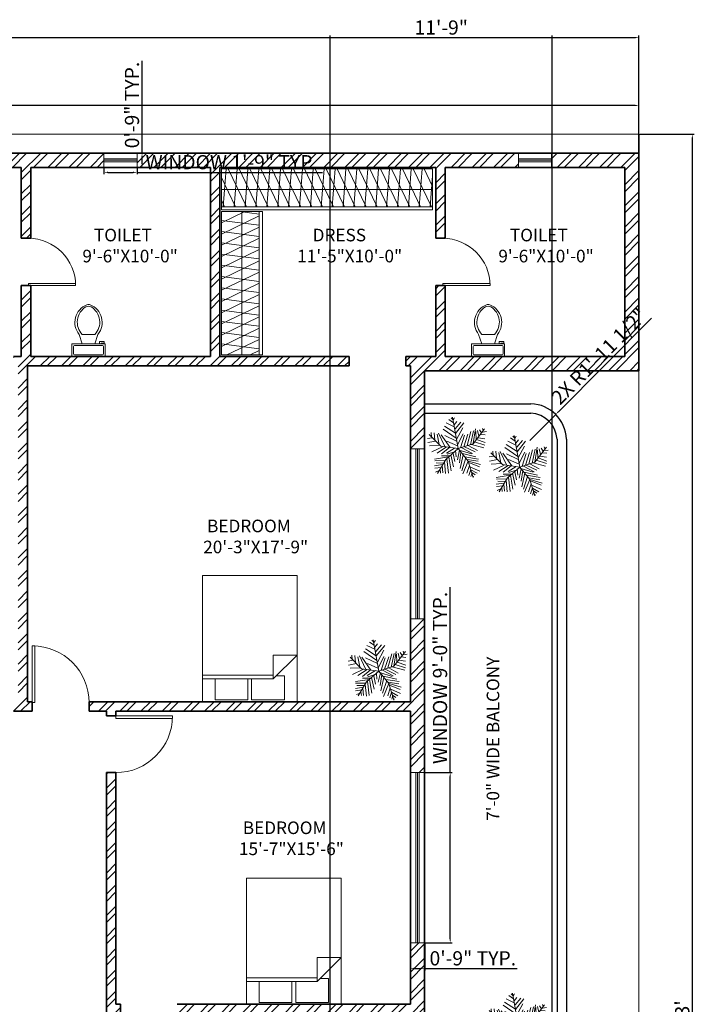
# Model space of a CAD drawing. Units: inches. Extents: x 155 to 1269, y 1260 to 2528.
# Tile 6 of 6: x 813 to 1242, y 1903 to 2528. Entities that reach past the tile are written whole.
import ezdxf

# ---------------------------------------------------------------- set-up
doc = ezdxf.new("R2010")
doc.units = ezdxf.units.IN
for name, color, linetype, lineweight in [('A-ANNO-DIMS', 2, 'Continuous', 18), ('A-AREA-IDEN', 7, 'Continuous', 18), ('A-DOOR', 3, 'Continuous', 18), ('A-FLOR-CASE', 9, 'Continuous', 18), ('A-FLOR-CASE-PATT', 252, 'Continuous', 13), ('A-FLOR-EDGE', 7, 'Continuous', 25), ('A-FLOR-FIXT', 9, 'Continuous', 18), ('A-FURN', 8, 'Continuous', 18), ('A-GLAZ', 244, 'Continuous', 18), ('A-WALL', 7, 'Continuous', 35), ('A-WALL-PATT', 252, 'Continuous', 13), ('C-PROP', 8, 'Continuous', 18), ('L-PLNT', 94, 'Continuous', 13)]:
    doc.layers.add(name, color=color, linetype=linetype, lineweight=lineweight)
doc.styles.get("Standard").update_dxf_attribs({"font": 'arial.ttf'})
doc.dimstyles.new('ISO-25', dxfattribs={"dimtxt": 9, "dimasz": 2.5, "dimexe": 1.25, "dimexo": 0.625, "dimtad": 1, "dimlunit": 3, "dimtxsty": 'Standard', "dimcen": 2.5, "dimadec": 0, "dimazin": 0, "dimtfac": 1, "dimtmove": 0, "dimatfit": 3, "dimfxl": 1, "dimarcsym": 0})

# ---------------------------------------------------------------- blocks, each defined once
blk = doc.blocks.new('*U3')
for p, q in [((0, 0), (0, -6)), ((40, 0), (40, -6))]:
    blk.add_line(p, q)
blk.add_lwpolyline([(0, 0), (0, 40), (1.75, 40), (1.75, 0)], close=True)
blk.add_arc((0, 0), 40, 0, 90)
blk = doc.blocks.new('*U4')
for p, q in [((-40, 0), (-40, 6)), ((0, 0), (0, 6))]:
    blk.add_line(p, q)
blk.add_lwpolyline([(0, 0), (0, -40), (-1.75, -40), (-1.75, 0)], close=True)
blk.add_arc((0, 0), 40, 180, 270)
blk = doc.blocks.new('*U2')
for p, q in [((0, 0), (0, -6)), ((-40, 0), (-40, -6))]:
    blk.add_line(p, q)
blk.add_lwpolyline([(0, 0), (0, 40), (-1.75, 40), (-1.75, 0)], close=True)
blk.add_arc((0, 0), 40, 90, 180)
blk = doc.blocks.new('Bed - Queen')
for p, q in [((0, -80.00003), (0, 0)), ((0, 0), (59.99999, 0)), ((59.99999, 0), (59.99999, -80.00003)), ((7.99999, -1.2), (28.79998, -1.2)), ((7.99999, -14.4), (7.99999, -1.2)), ((28.79998, -1.2), (28.79998, -14.4)), ((31.19999, -1.2), (51.99999, -1.2)), ((31.19999, -14.4), (31.19999, -1.2)), ((51.99999, -1.2), (51.99999, -16.4)), ((0, -14.4), (44.8, -14.4)), ((44.8, -16.8), (0, -16.8)), ((59.99999, -29.6), (44.8, -14.4)), ((44.8, -14.4), (44.8, -29.6)), ((51.99999, -16.4), (46.79936, -16.4)), ((44.8, -29.6), (59.99999, -29.6)), ((59.99999, -80.00003), (0, -80.00003))]:
    blk.add_line(p, q)
blk = doc.blocks.new('*U8')
for p, q in [((9.5, -6), (9.5, -2)), ((-10, -8.5), (-8, -8.5)), ((-10, -9.5), (-10, -8.5)), ((-7, -9.5), (-10, -9.5)), ((-8, -8.5), (-8, -8)), ((-7, -8), (-7, -9.5)), ((-4, -8), (-6, -14)), ((4, -8), (6, -14)), ((4, -14), (-4, -14))]:
    blk.add_line(p, q)
blk.add_lwpolyline([(10.5, -8), (10.5, 0), (-10.5, 0), (-10.5, -8)], close=True)
for points in [[(-9.5, -2), (-9.5, -6)], [(8.5, -1), (-8.5, -1)], [(-8.5, -7), (8.5, -7)]]:
    blk.add_lwpolyline(points)
for centre, radius, start, end in [((-8.62, -1.88), 0.884, 81.8699, 188.1301), ((-8.62, -6.12), 0.884, 171.8699, 278.1301), ((8.62, -1.88), 0.884, 351.8699, 98.1301), ((8.62, -6.12), 0.884, 261.8699, 8.1301), ((3.52, -21.58), 12.17, 141.46911, 247.97143), ((4.2, -21.82), 11.33, 136.36773, 238.94682), ((-3.52, -21.58), 12.17, 292.02843, 38.53071), ((-4.2, -21.82), 11.33, 301.05301, 43.63209), ((0, -27.88), 4, 245.73182, 294.26817), ((0, -29), 4, 254.86053, 285.13947)]:
    blk.add_arc(centre, radius, start, end)
blk = doc.blocks.new('*U11')
for p, q in [((-10.186, 53.64), (-13.084, 55.962)), ((0, 0), (-10.5, 57)), ((-9.099, 51.782), (-6.563, 55.962)), ((-5.114, 28.097), (-24.676, 40.636)), ((-7.288, 39.707), (-21.778, 46.673)), ((-8.737, 47.138), (-17.069, 52.711)), ((-7.65, 43.423), (-2.578, 49.46)), ((-5.839, 35.992), (4.667, 48.067)), ((-5.114, 27.632), (10.463, 46.673)), ((-2.941, 16.486), (8.652, 37.85)), ((27, 9), (48, 36)), ((27.127, 9.056), (31.112, 35.992)), ((44.153, 36.456), (45.239, 32.741)), ((-47.498, 19.737), (-55.83, 18.344)), ((-31.5, 4.5), (-52.5, 25.5)), ((-48.585, 21.131), (-49.309, 29.026)), ((-43.513, 28.561), (-42.427, 15.558)), ((-38.442, 26.239), (-34.819, 7.663)), ((-35.544, 28.097), (-24.314, 3.947)), ((-14.533, 2.09), (-30.834, 25.31)), ((-3.665, 19.273), (-27.574, 35.527)), ((-24.314, 23.917), (-2.941, 13.7)), ((-1.129, 6.734), (9.014, 26.704)), ((3.942, 1.625), (11.187, 24.381)), ((10.101, 3.483), (17.708, 26.239)), ((16.259, 5.805), (23.142, 31.348)), ((22.055, 7.198), (27.489, 32.277)), ((31.836, 30.883), (32.561, 16.486)), ((35.096, 32.741), (37.27, 22.524)), ((36.183, 19.737), (48.137, 17.88)), ((38.719, 34.134), (41.979, 28.561)), ((40.53, 25.775), (48.862, 24.846)), ((43.791, 29.954), (51.036, 30.883)), ((-40.615, 13.7), (-55.105, 10.913)), ((-33.37, 6.269), (-52.207, 5.34)), ((-28.299, 3.483), (-47.86, -5.805)), ((-21.416, 3.018), (-38.079, -8.128)), ((0, 0), (-31.5, 4.5)), ((-15.982, 2.09), (-30.11, -9.521)), ((0, 0), (-22.5, -19.5)), ((-6.563, 1.161), (-21.416, -8.128)), ((-20.691, 13.7), (-1.129, 4.876)), ((0, 0), (27, 9)), ((0, 0), (18, -22.5)), ((6.478, 1.625), (26.04, -8.592)), ((11.187, 3.483), (30.749, -5.805)), ((18.07, 5.805), (35.096, -3.483)), ((24.229, 7.663), (46.688, 1.625)), ((29.662, 12.307), (48.137, 6.269)), ((33.285, 16.486), (48.862, 10.913)), ((-17.431, -15.094), (-42.789, -18.809)), ((-15.257, -12.772), (-30.11, -12.772)), ((-6.563, -5.805), (-19.967, -9.985)), ((-17.069, -15.094), (-12.721, -40.172)), ((-13.446, -11.378), (-8.737, -32.741)), ((-9.461, -8.592), (-6.201, -23.453)), ((-4.752, -3.483), (-3.665, -14.629)), ((2.493, -3.019), (-1.491, -20.202)), ((1.769, -2.555), (24.229, -9.521)), ((5.029, -6.27), (2.131, -25.775)), ((9.014, -11.378), (3.58, -35.992)), ((14.085, -16.951), (6.478, -40.172)), ((7.565, -9.056), (32.198, -14.629)), ((12.274, -15.094), (36.907, -18.809)), ((-28.299, -29.026), (-42.789, -31.348)), ((-24.314, -21.596), (-42.427, -22.06)), ((-30.834, -34.135), (-42.427, -35.528)), ((-26.849, -26.24), (-40.253, -25.775)), ((-22.5, -19.5), (-37.5, -45)), ((-29.023, -30.884), (-27.936, -43.887)), ((-25.038, -23.918), (-22.865, -45.281)), ((-20.691, -18.345), (-17.793, -44.352)), ((18.07, -22.524), (8.289, -45.745)), ((20.244, -30.419), (15.897, -44.816)), ((16.259, -19.738), (36.183, -22.989)), ((18, -22.5), (27, -52.5)), ((18.433, -22.524), (40.53, -29.026)), ((19.157, -25.311), (38.719, -33.206)), ((21.331, -32.741), (39.081, -40.636)), ((-34.457, -39.708), (-40.978, -42.494)), ((-32.646, -36.921), (-31.921, -44.352)), ((22.78, -37.85), (19.519, -48.532)), ((22.78, -38.314), (34.372, -44.816)), ((24.591, -45.745), (23.142, -50.854)), ((24.591, -43.423), (30.749, -47.603)), ((26.764, -49.925), (28.213, -50.854))]:
    blk.add_line(p, q)
blk = doc.blocks.new('*D12')
at = {"layer": 'A-ANNO-DIMS', "color": 0, "lineweight": -2, "transparency": 16777216}
for p, q in [((227.4, 2455.81), (227.4, 2474.72)), ((1206.4, 2455.81), (1206.4, 2474.72)), ((1203.9, 2473.47), (229.9, 2473.47))]:
    blk.add_line(p, q, dxfattribs=at)
at = {"layer": 'A-ANNO-DIMS', "color": 0, "transparency": 16777216}
for points in [[(229.9, 2473.89), (229.9, 2473.06), (227.4, 2473.47)], [(1203.9, 2473.89), (1203.9, 2473.06), (1206.4, 2473.47)]]:
    blk.add_solid(points, dxfattribs=at)
at = {"layer": 'Defpoints', "color": 0, "transparency": 16777216}
for p in [(227.4, 2473.47), (227.4, 2455.18), (1206.4, 2455.18)]:
    blk.add_point(p, dxfattribs=at)
at = {"layer": 'A-ANNO-DIMS', "color": 0, "transparency": 16777216, "insert": (716.9, 2478.69), "char_height": 9, "attachment_point": 5}
blk.add_mtext('81\'-7"', dxfattribs=at)
blk = doc.blocks.new('*D13')
at = {"layer": 'A-ANNO-DIMS', "color": 0, "lineweight": -2, "transparency": 16777216}
for p, q in [((1207.02, 2455.18), (1241.52, 2455.18)), ((1240.27, 1341.68), (1240.27, 2452.68)), ((1207.02, 1339.18), (1241.52, 1339.18))]:
    blk.add_line(p, q, dxfattribs=at)
at = {"layer": 'A-ANNO-DIMS', "color": 0, "transparency": 16777216}
for points in [[(1239.85, 2452.68), (1240.68, 2452.68), (1240.27, 2455.18)], [(1239.85, 1341.68), (1240.68, 1341.68), (1240.27, 1339.18)]]:
    blk.add_solid(points, dxfattribs=at)
at = {"layer": 'Defpoints', "color": 0, "transparency": 16777216}
for p in [(1206.4, 2455.18), (1240.27, 2455.18), (1206.4, 1339.18)]:
    blk.add_point(p, dxfattribs=at)
at = {"layer": 'A-ANNO-DIMS', "color": 0, "transparency": 16777216, "insert": (1235.04, 1897.18), "char_height": 9, "attachment_point": 5, "rotation": 90}
blk.add_mtext("93'", dxfattribs=at)
blk = doc.blocks.new('WIN-21IN')
for p, q in [((21, 5.5), (0, 5.5)), ((21, 4.5), (0, 4.5)), ((21, 3.5), (0, 3.5))]:
    blk.add_line(p, q)
blk.add_lwpolyline([(0, 9), (21, 9), (21, 0), (0, 0)], close=True)
blk = doc.blocks.new('WIN-108IN')
for p, q in [((3.5, 108), (3.5, 0)), ((4.5, 108), (4.5, 0)), ((5.5, 108), (5.5, 0))]:
    blk.add_line(p, q)
blk.add_lwpolyline([(9, 108), (9, 0), (0, 0), (0, 108)], close=True)
blk = doc.blocks.new('*D24')
at = {"layer": 'A-ANNO-DIMS', "color": 0, "lineweight": -2, "transparency": 16777216}
for p, q in [((866.9, 2433.56), (866.9, 2429.78)), ((869.4, 2431.03), (885.4, 2431.03)), ((887.9, 2433.56), (887.9, 2429.78)), ((887.9, 2431.03), (1005.53, 2431.03))]:
    blk.add_line(p, q, dxfattribs=at)
at = {"layer": 'A-ANNO-DIMS', "color": 0, "transparency": 16777216}
for points in [[(869.4, 2431.45), (869.4, 2430.61), (866.9, 2431.03)], [(885.4, 2431.45), (885.4, 2430.61), (887.9, 2431.03)]]:
    blk.add_solid(points, dxfattribs=at)
at = {"layer": 'Defpoints', "color": 0, "transparency": 16777216}
for p in [(866.9, 2434.18), (887.9, 2434.18), (887.9, 2431.03)]:
    blk.add_point(p, dxfattribs=at)
at = {"layer": 'A-ANNO-DIMS', "color": 0, "transparency": 16777216, "insert": (947.97, 2436.31), "char_height": 9, "attachment_point": 5}
blk.add_mtext('WINDOW 1\'-9" TYP.', dxfattribs=at)
blk = doc.blocks.new('*D25')
at = {"layer": 'A-ANNO-DIMS', "color": 0, "lineweight": -2, "transparency": 16777216}
for p, q in [((891.05, 2443.18), (891.05, 2501.79)), ((888.52, 2443.18), (892.3, 2443.18)), ((891.05, 2436.68), (891.05, 2440.68)), ((888.52, 2434.18), (892.3, 2434.18))]:
    blk.add_line(p, q, dxfattribs=at)
at = {"layer": 'A-ANNO-DIMS', "color": 0, "transparency": 16777216}
for points in [[(890.63, 2440.68), (891.46, 2440.68), (891.05, 2443.18)], [(890.63, 2436.68), (891.46, 2436.68), (891.05, 2434.18)]]:
    blk.add_solid(points, dxfattribs=at)
at = {"layer": 'Defpoints', "color": 0, "transparency": 16777216}
for p in [(887.9, 2443.18), (891.05, 2443.18), (887.9, 2434.18)]:
    blk.add_point(p, dxfattribs=at)
at = {"layer": 'A-ANNO-DIMS', "color": 0, "transparency": 16777216, "insert": (885.83, 2473.74), "char_height": 9, "attachment_point": 5, "rotation": 90}
blk.add_mtext('0\'-9" TYP.', dxfattribs=at)
blk = doc.blocks.new('*D28')
at = {"layer": 'A-ANNO-DIMS', "color": 0, "lineweight": -2, "transparency": 16777216}
for p, q in [((1086.6, 2050.18), (1086.6, 2167.82)), ((1071.02, 2050.18), (1087.85, 2050.18)), ((1086.6, 1944.68), (1086.6, 2047.68)), ((1071.02, 1942.18), (1087.85, 1942.18))]:
    blk.add_line(p, q, dxfattribs=at)
at = {"layer": 'A-ANNO-DIMS', "color": 0, "transparency": 16777216}
for points in [[(1086.18, 2047.68), (1087.01, 2047.68), (1086.6, 2050.18)], [(1086.18, 1944.68), (1087.01, 1944.68), (1086.6, 1942.18)]]:
    blk.add_solid(points, dxfattribs=at)
at = {"layer": 'Defpoints', "color": 0, "transparency": 16777216}
for p in [(1070.4, 2050.18), (1086.6, 2050.18), (1070.4, 1942.18)]:
    blk.add_point(p, dxfattribs=at)
at = {"layer": 'A-ANNO-DIMS', "color": 0, "transparency": 16777216, "insert": (1081.32, 2110.25), "char_height": 9, "attachment_point": 5, "rotation": 90}
blk.add_mtext('WINDOW 9\'-0" TYP.', dxfattribs=at)
blk = doc.blocks.new('*D29')
at = {"layer": 'A-ANNO-DIMS', "color": 0, "lineweight": -2, "transparency": 16777216}
for p, q in [((1061.4, 1941.56), (1061.4, 1924.73)), ((1070.4, 1941.56), (1070.4, 1924.73)), ((1063.9, 1925.98), (1067.9, 1925.98)), ((1070.4, 1925.98), (1129.01, 1925.98))]:
    blk.add_line(p, q, dxfattribs=at)
at = {"layer": 'A-ANNO-DIMS', "color": 0, "transparency": 16777216}
for points in [[(1063.9, 1926.4), (1063.9, 1925.56), (1061.4, 1925.98)], [(1067.9, 1926.4), (1067.9, 1925.56), (1070.4, 1925.98)]]:
    blk.add_solid(points, dxfattribs=at)
at = {"layer": 'Defpoints', "color": 0, "transparency": 16777216}
for p in [(1061.4, 1942.18), (1070.4, 1942.18), (1070.4, 1925.98)]:
    blk.add_point(p, dxfattribs=at)
at = {"layer": 'A-ANNO-DIMS', "color": 0, "transparency": 16777216, "insert": (1100.95, 1931.2), "char_height": 9, "attachment_point": 5}
blk.add_mtext('0\'-9" TYP.', dxfattribs=at)
blk = doc.blocks.new('*D42')
at = {"layer": 'A-ANNO-DIMS', "color": 0, "lineweight": -2, "transparency": 16777216}
for p, q in [((293.4, 2443.81), (293.4, 2517.78)), ((1206.4, 2443.81), (1206.4, 2517.78)), ((295.9, 2516.53), (1203.9, 2516.53))]:
    blk.add_line(p, q, dxfattribs=at)
at = {"layer": 'A-ANNO-DIMS', "color": 0, "transparency": 16777216}
for points in [[(295.9, 2516.95), (295.9, 2516.11), (293.4, 2516.53)], [(1203.9, 2516.95), (1203.9, 2516.11), (1206.4, 2516.53)]]:
    blk.add_solid(points, dxfattribs=at)
at = {"layer": 'Defpoints', "color": 0, "transparency": 16777216}
for p in [(1206.4, 2516.53), (293.4, 2443.18), (1206.4, 2443.18)]:
    blk.add_point(p, dxfattribs=at)
at = {"layer": 'A-ANNO-DIMS', "color": 0, "transparency": 16777216, "insert": (749.9, 2521.75), "char_height": 9, "attachment_point": 5}
blk.add_mtext('76\'-1"', dxfattribs=at)
blk = doc.blocks.new('*D45')
at = {"layer": 'A-ANNO-DIMS', "color": 0, "lineweight": -2, "transparency": 16777216}
for p, q in [((1010.4, 1819.81), (1010.4, 2517.78)), ((1151.4, 1819.81), (1151.4, 2517.78)), ((1012.9, 2516.53), (1148.9, 2516.53))]:
    blk.add_line(p, q, dxfattribs=at)
at = {"layer": 'A-ANNO-DIMS', "color": 0, "transparency": 16777216}
for points in [[(1012.9, 2516.95), (1012.9, 2516.11), (1010.4, 2516.53)], [(1148.9, 2516.95), (1148.9, 2516.11), (1151.4, 2516.53)]]:
    blk.add_solid(points, dxfattribs=at)
at = {"layer": 'Defpoints', "color": 0, "transparency": 16777216}
for p in [(1151.4, 2516.53), (1010.4, 1819.18), (1151.4, 1819.18)]:
    blk.add_point(p, dxfattribs=at)
at = {"layer": 'A-ANNO-DIMS', "color": 0, "transparency": 16777216, "insert": (1080.9, 2521.75), "char_height": 9, "attachment_point": 5}
blk.add_mtext('11\'-9"', dxfattribs=at)
blk = doc.blocks.new('*D49')
at = {"layer": 'A-ANNO-DIMS', "color": 0, "lineweight": -2, "transparency": 16777216}
for p, q in [((1214.34, 2338.57), (1155.3, 2279.18)), ((1137.09, 2260.87), (1153.54, 2277.41))]:
    blk.add_line(p, q, dxfattribs=at)
at = {"layer": 'A-ANNO-DIMS', "color": 0, "transparency": 16777216}
blk.add_solid([(1155, 2279.48), (1155.6, 2278.89), (1153.54, 2277.41)], dxfattribs=at)
at = {"layer": 'Defpoints', "color": 0, "transparency": 16777216}
for p in [(1153.54, 2277.41), (1137.09, 2260.87)]:
    blk.add_point(p, dxfattribs=at)
at = {"layer": 'A-ANNO-DIMS', "color": 0, "transparency": 16777216, "insert": (1181.96, 2313.49), "char_height": 9, "attachment_point": 5, "rotation": 45.16583}
blk.add_mtext('2X R1\'-11 1/2"', dxfattribs=at)

msp = doc.modelspace()

# ---------------------------------------------------------------- hatches: boundary and pattern name
at = {"layer": 'A-FLOR-CASE-PATT'}
h = msp.add_hatch(dxfattribs=at)
h.set_pattern_fill('ANSI31', color=256, scale=1.9617, angle=70.6537, style=0)
h.paths.add_polyline_path([(941.397, 2409.181), (1075.397, 2409.181), (1075.397, 2433.181), (941.397, 2433.181)])
h = msp.add_hatch(dxfattribs=at)
h.set_pattern_fill('ANSI31', color=256, scale=2.16999, angle=40.6661, style=0)
h.paths.add_polyline_path([(941.397, 2409.181), (1075.397, 2409.181), (1075.397, 2433.181), (941.397, 2433.181)])
h = msp.add_hatch(dxfattribs=at)
h.set_pattern_fill('ANSI31', color=256, scale=2.02178, angle=-19.2697, style=0)
h.paths.add_polyline_path([(941.397, 2315.181), (965.397, 2315.181), (965.397, 2406.181), (941.397, 2406.181)])
h = msp.add_hatch(dxfattribs=at)
h.set_pattern_fill('ANSI31', color=256, scale=2.225716, angle=127.6207, style=0)
h.paths.add_polyline_path([(941.397, 2315.181), (965.397, 2315.181), (965.397, 2406.181), (941.397, 2406.181)])
at = {"layer": 'A-WALL-PATT'}
h = msp.add_hatch(dxfattribs=at)
h.set_pattern_fill('ANSI32', color=256)
h.paths.add_polyline_path([(614.897, 1534.181), (593.397, 1534.181), (593.397, 1555.181), (589.397, 1555.181), (589.397, 1534.181), (517.397, 1534.181), (517.397, 1555.181), (511.397, 1555.181), (511.397, 1495.181), (488.631, 1495.181), (488.631, 1486.181), (517.397, 1486.181), (517.397, 1525.181), (614.897, 1525.181)])
h.paths.add_polyline_path([(440.631, 1495.181), (344.954, 1495.181), (344.954, 1486.181), (440.631, 1486.181)])
h.paths.add_polyline_path([(323.954, 1495.181), (302.397, 1495.181), (302.397, 1625.863), (332.397, 1625.863), (332.397, 1631.863), (302.397, 1631.863), (302.397, 1634.984), (293.397, 1634.984), (293.397, 1486.181), (323.954, 1486.181)])
h.paths.add_polyline_path([(302.397, 1753.181), (386.397, 1753.181), (386.397, 1726.181), (392.397, 1726.181), (392.397, 1753.181), (511.397, 1753.181), (511.397, 1693.181), (392.397, 1693.181), (392.397, 1696.181), (386.397, 1696.181), (386.397, 1693.181), (368.397, 1693.181), (368.397, 1687.181), (511.397, 1687.181), (511.397, 1663.181), (517.397, 1663.181), (517.397, 1891.181), (539.397, 1891.181), (539.397, 1897.181), (517.397, 1897.181), (517.397, 2050.181), (511.397, 2050.181), (511.397, 1903.181), (374.397, 1903.181), (374.397, 1897.181), (410.397, 1897.181), (410.397, 1843.181), (416.397, 1843.181), (416.397, 1897.181), (511.397, 1897.181), (511.397, 1759.181), (416.397, 1759.181), (416.397, 1813.181), (410.397, 1813.181), (410.397, 1759.181), (302.397, 1759.181), (302.397, 1897.181), (338.397, 1897.181), (338.397, 1903.181), (302.397, 1903.181), (302.397, 1935.29), (293.397, 1935.29), (293.397, 1682.984), (302.397, 1682.984), (302.397, 1687.181), (338.397, 1687.181), (338.397, 1693.181), (302.397, 1693.181)])
h.paths.add_polyline_path([(645.397, 1897.181), (623.397, 1897.181), (623.397, 1891.181), (645.397, 1891.181)])
h.paths.add_polyline_path([(678.397, 1897.181), (669.397, 1897.181), (669.397, 1891.181), (678.397, 1891.181)])
h.paths.add_polyline_path([(696.397, 1897.181), (687.397, 1897.181), (687.397, 1891.181), (696.397, 1891.181)])
h.paths.add_polyline_path([(714.397, 1897.181), (705.397, 1897.181), (705.397, 1891.181), (714.397, 1891.181)])
h.paths.add_polyline_path([(732.397, 1897.181), (723.397, 1897.181), (723.397, 1891.181), (732.397, 1891.181)])
h.paths.add_polyline_path([(302.397, 2033.891), (293.397, 2033.891), (293.397, 1959.29), (302.397, 1959.29)], flags=17)
h.paths.add_polyline_path([(302.397, 2089.181), (511.397, 2089.181), (511.397, 2086.181), (517.397, 2086.181), (517.397, 2089.181), (527.397, 2089.181), (527.397, 2095.181), (302.397, 2095.181), (302.397, 2145.471), (293.397, 2145.471), (293.397, 2057.891), (302.397, 2057.891)])
h.paths.add_polyline_path([(773.397, 2095.181), (572.397, 2095.181), (572.397, 2308.181), (613.397, 2308.181), (613.397, 2443.181), (557.897, 2443.181), (557.897, 2434.181), (604.397, 2434.181), (604.397, 2314.181), (490.397, 2314.181), (490.397, 2359.181), (484.397, 2359.181), (484.397, 2314.181), (374.397, 2314.181), (374.397, 2308.181), (566.397, 2308.181), (566.397, 2095.181), (563.397, 2095.181), (563.397, 2089.181), (773.397, 2089.181)])
h.paths.add_polyline_path([(1070.397, 2147.681), (1061.397, 2147.681), (1061.397, 2095.181), (857.397, 2095.181), (857.397, 2089.181), (868.397, 2089.181), (868.397, 2086.181), (874.397, 2086.181), (874.397, 2089.181), (1061.397, 2089.181), (1061.397, 2050.181), (1070.397, 2050.181)])
h.paths.add_polyline_path([(821.397, 2095.181), (818.397, 2095.181), (818.397, 2308.181), (1022.397, 2308.181), (1022.397, 2314.181), (940.397, 2314.181), (940.397, 2434.181), (1077.397, 2434.181), (1077.397, 2389.181), (1083.397, 2389.181), (1083.397, 2434.181), (1129.897, 2434.181), (1129.897, 2443.181), (887.897, 2443.181), (887.897, 2434.181), (934.397, 2434.181), (934.397, 2314.181), (820.397, 2314.181), (820.397, 2359.181), (814.397, 2359.181), (814.397, 2314.181), (809.397, 2314.181), (809.397, 2308.181), (812.397, 2308.181), (812.397, 2095.181), (809.397, 2095.181), (809.397, 2089.181), (821.397, 2089.181)])
h.paths.add_polyline_path([(874.397, 2050.181), (868.397, 2050.181), (868.397, 1741.181), (877.397, 1741.181), (877.397, 1747.181), (892.397, 1747.181), (892.397, 1753.181), (874.397, 1753.181), (874.397, 1819.181), (940.397, 1819.181), (940.397, 1753.181), (922.397, 1753.181), (922.397, 1747.181), (946.397, 1747.181), (946.397, 1819.181), (1151.397, 1819.181), (1151.397, 1683.181), (931.397, 1683.181), (931.397, 1677.181), (1064.397, 1677.181), (1064.397, 1495.181), (877.397, 1495.181), (877.397, 1638.181), (868.397, 1638.181), (868.397, 1534.181), (796.397, 1534.181), (796.397, 1555.181), (792.397, 1555.181), (792.397, 1534.181), (770.897, 1534.181), (770.897, 1525.181), (868.397, 1525.181), (868.397, 1486.181), (1073.397, 1486.181), (1073.397, 1677.181), (1160.397, 1677.181), (1160.397, 1825.181), (1070.397, 1825.181), (1070.397, 1942.181), (1061.397, 1942.181), (1061.397, 1903.181), (913.397, 1903.181), (913.397, 1897.181), (1061.397, 1897.181), (1061.397, 1825.181), (957.406, 1825.181), (957.406, 1861.181), (951.406, 1861.181), (951.406, 1825.181), (874.397, 1825.181), (874.397, 1897.181), (877.397, 1897.181), (877.397, 1903.181), (874.397, 1903.181)])
h.paths.add_polyline_path([(1070.397, 2305.181), (1206.397, 2305.181), (1206.397, 2443.181), (1150.897, 2443.181), (1150.897, 2434.181), (1197.397, 2434.181), (1197.397, 2314.181), (1083.397, 2314.181), (1083.397, 2359.181), (1077.397, 2359.181), (1077.397, 2314.181), (1058.397, 2314.181), (1058.397, 2308.181), (1061.397, 2308.181), (1061.397, 2255.681), (1070.397, 2255.681)])
h.paths.add_polyline_path([(866.897, 2443.181), (673.397, 2443.181), (673.397, 2308.181), (773.397, 2308.181), (773.397, 2314.181), (682.397, 2314.181), (682.397, 2434.181), (814.397, 2434.181), (814.397, 2389.181), (818.897, 2389.181), (820.397, 2389.181), (820.397, 2434.181), (866.897, 2434.181)])
h.paths.add_polyline_path([(536.897, 2443.181), (293.397, 2443.181), (293.397, 2253.471), (302.397, 2253.471), (302.397, 2308.181), (338.397, 2308.181), (338.397, 2314.181), (302.397, 2314.181), (302.397, 2434.181), (484.397, 2434.181), (484.397, 2389.181), (490.397, 2389.181), (490.397, 2434.181), (536.897, 2434.181)])

# ---------------------------------------------------------------- linework, layer by layer
at = {"layer": 'A-FLOR-CASE'}
for p, q in [((941.397, 2433.181), (1075.397, 2433.181)), ((941.397, 2433.181), (941.397, 2407.181)), ((1075.397, 2433.181), (1075.397, 2407.181)), ((941.397, 2420.181), (1075.397, 2420.181)), ((941.397, 2409.181), (1075.397, 2409.181)), ((941.397, 2407.181), (1075.397, 2407.181)), ((941.397, 2406.181), (967.397, 2406.181)), ((941.397, 2406.181), (941.397, 2315.181)), ((954.397, 2406.181), (954.397, 2315.181)), ((965.397, 2406.181), (965.397, 2315.181)), ((967.397, 2406.181), (967.397, 2315.181)), ((941.397, 2315.181), (967.397, 2315.181))]:
    msp.add_line(p, q, dxfattribs=at)
at = {"layer": 'A-FLOR-EDGE'}
for p, q in [((1070.397, 2284.181), (1137.877, 2284.181)), ((1070.397, 2278.181), (1137.769, 2278.181)), ((1154.397, 2261.664), (1154.397, 1858.359)), ((1160.397, 2261.791), (1160.397, 1858.209))]:
    msp.add_line(p, q, dxfattribs=at)
for radius, start, end in [(23.321, 2.254968, 88.076393), (17.321, 2.616598, 87.767917)]:
    msp.add_arc((1137.094, 2260.873), radius, start, end, dxfattribs=at)
at = {"layer": 'A-WALL'}
for p, q in [((1206.397, 2455.181), (1206.397, 2305.181)), ((673.397, 2443.181), (1206.397, 2443.181)), ((682.397, 2434.181), (814.397, 2434.181)), ((814.397, 2434.181), (814.397, 2389.181)), ((820.397, 2434.181), (820.397, 2389.181)), ((820.397, 2434.181), (934.397, 2434.181)), ((934.397, 2434.181), (934.397, 2314.181)), ((940.397, 2434.181), (940.397, 2314.181)), ((940.397, 2434.181), (1077.397, 2434.181)), ((1077.397, 2434.181), (1077.397, 2389.181)), ((1083.397, 2434.181), (1083.397, 2389.181)), ((1083.397, 2434.181), (1197.397, 2434.181)), ((1197.397, 2434.181), (1197.397, 2314.181)), ((820.397, 2389.181), (814.397, 2389.181)), ((1083.397, 2389.181), (1077.397, 2389.181)), ((820.397, 2359.181), (814.397, 2359.181)), ((814.397, 2359.181), (814.397, 2314.181)), ((820.397, 2359.181), (820.397, 2314.181)), ((1083.397, 2359.181), (1077.397, 2359.181)), ((1077.397, 2359.181), (1077.397, 2314.181)), ((1083.397, 2359.181), (1083.397, 2314.181)), ((809.397, 2314.181), (814.397, 2314.181)), ((820.397, 2314.181), (934.397, 2314.181)), ((940.397, 2314.181), (1022.397, 2314.181)), ((1022.397, 2308.181), (1022.397, 2314.181)), ((1058.397, 2308.181), (1058.397, 2314.181)), ((1058.397, 2314.181), (1077.397, 2314.181)), ((1083.397, 2314.181), (1197.397, 2314.181)), ((818.397, 2308.181), (818.397, 2095.181)), ((818.397, 2308.181), (1022.397, 2308.181)), ((1058.397, 2308.181), (1061.397, 2308.181)), ((1061.397, 2308.181), (1061.397, 2095.181)), ((1070.397, 2305.181), (1070.397, 1825.181)), ((1070.397, 2305.181), (1206.397, 2305.181)), ((818.397, 2095.181), (821.397, 2095.181)), ((821.397, 2095.181), (821.397, 2089.181)), ((857.397, 2095.181), (857.397, 2089.181)), ((857.397, 2095.181), (1061.397, 2095.181)), ((809.397, 2089.181), (821.397, 2089.181)), ((857.397, 2089.181), (868.397, 2089.181)), ((868.397, 2089.181), (868.397, 2086.181)), ((874.397, 2089.181), (874.397, 2086.181)), ((874.397, 2089.181), (1061.397, 2089.181)), ((1061.397, 2089.181), (1061.397, 1903.181)), ((868.397, 2086.181), (874.397, 2086.181)), ((868.397, 2050.181), (874.397, 2050.181)), ((868.397, 2050.181), (868.397, 1741.181)), ((874.397, 2050.181), (874.397, 1903.181)), ((874.397, 1903.181), (877.397, 1903.181)), ((877.397, 1897.181), (877.397, 1903.181)), ((913.397, 1903.181), (1061.397, 1903.181))]:
    msp.add_line(p, q, dxfattribs=at)
at = {"layer": 'C-PROP'}
for p, q in [((227.397, 2455.181), (1206.397, 2455.181)), ((1206.397, 2305.181), (1206.397, 1339.181))]:
    msp.add_line(p, q, dxfattribs=at)

# ---------------------------------------------------------------- block references
at = {"layer": 'A-DOOR'}
for name, p, xscale, yscale, zscale, rotation in [('*U2', (818.897, 2359.181), 0.7500000000000114, 0.7500000000000114, 0.7500000000000114, 270), ('*U2', (1081.897, 2359.181), 0.7500000000000114, 0.7500000000000114, 0.7500000000000114, 270), ('*U4', (874.397, 2086.181), 0.9, 0.9, 0.9, 90)]:
    msp.add_blockref(name, p, dxfattribs=dict(at, xscale=xscale, yscale=yscale, zscale=zscale, rotation=rotation))
at = {"layer": 'A-DOOR', "xscale": 0.9, "yscale": 0.9, "zscale": 0.9}
msp.add_blockref('*U3', (821.397, 2094.581), dxfattribs=at)
at = {"layer": 'A-FLOR-FIXT', "rotation": 180}
for p in [(857.088, 2314.181), (1110.659, 2314.181)]:
    msp.add_blockref('*U8', p, dxfattribs=at)
at = {"layer": 'A-FURN', "xscale": -1, "rotation": 180}
for p in [(929.397, 2095.181), (957.397, 1903.181)]:
    msp.add_blockref('Bed - Queen', p, dxfattribs=at)
at = {"layer": 'A-GLAZ'}
for name, p in [('WIN-21IN', (866.897, 2434.181)), ('WIN-21IN', (1129.897, 2434.181)), ('WIN-108IN', (1061.397, 2147.681)), ('WIN-108IN', (1061.397, 1942.181))]:
    msp.add_blockref(name, p, dxfattribs=at)
at = {"layer": 'L-PLNT', "xscale": 0.3495173552522817, "yscale": 0.3495173552522817, "zscale": 0.3495173552522817}
for p in [(1091.697, 2255.73), (1130.834, 2244.074), (1041.395, 2114.546), (1129.772, 1890.256)]:
    msp.add_blockref('*U11', p, dxfattribs=at)

# ---------------------------------------------------------------- texts
at = {"layer": 'A-AREA-IDEN', "char_height": 8, "attachment_point": 1}
for s, width, insert in [('   TOILET\\P9\'-6"X10\'-0"', 56.71156, (853.199, 2395.252)), ('    DRESS\\P11\'-5"X10\'-0"', 61.72868, (989.536, 2395.252)), ('   TOILET\\P9\'-6"X10\'-0"', 56.71156, (1117.167, 2395.252)), (' BEDROOM\\P20\'-3"X17\'-9"', 61.72868, (929.875, 2210.676)), (' BEDROOM\\P15\'-7"X15\'-6"', 61.72868, (952.546, 2019.18))]:
    msp.add_mtext_dynamic_manual_height_columns(s, width=width, gutter_width=12.5, heights=[0], dxfattribs=dict(at, insert=insert))
at = {"layer": 'A-AREA-IDEN', "insert": (1109.739, 2019.55), "char_height": 8, "attachment_point": 1, "rotation": 90}
msp.add_mtext_dynamic_manual_height_columns('7\'-0" WIDE BALCONY', width=110.88305, gutter_width=12.5, heights=[0], dxfattribs=at)

# ---------------------------------------------------------------- dimensions: what is measured, and where the dimension line sits
at = {"layer": 'A-ANNO-DIMS'}
for base, p1, p2, override, picture, middle in [((1206.397, 2516.531), (293.397, 2443.181), (1206.397, 2443.181), {"dimdec": 1, "dimlfac": 1, "dimrnd": 0, "dimzin": 1, "dimdsep": 46, "dimlunit": 4, "dimfrac": 2}, '*D42', (749.897, 2521.751)), ((1151.397, 2516.531), (1010.397, 1819.181), (1151.397, 1819.181), {"dimdec": 1, "dimlfac": 1, "dimrnd": 0, "dimzin": 1, "dimdsep": 46, "dimlunit": 4, "dimfrac": 2}, '*D45', (1080.897, 2521.751)), ((227.397, 2473.473), (1206.397, 2455.181), (227.397, 2455.181), {"dimclrd": 0, "dimclre": 0, "dimclrt": 0}, '*D12', (716.897, 2478.693))]:
    dim = msp.add_linear_dim(base=base, p1=p1, p2=p2, dimstyle='ISO-25', override=override, dxfattribs=at)
    dim.commit()
    dim.dimension.update_dxf_attribs({"geometry": picture, "text_midpoint": middle})
for base, p1, p2, text, picture, middle in [((891.047, 2443.181), (887.897, 2434.181), (887.897, 2443.181), '<> TYP.', '*D25', (885.827, 2473.736)), ((1086.597, 2050.181), (1070.397, 1942.181), (1070.397, 2050.181), 'WINDOW <> TYP.', '*D28', (1081.316, 2110.25))]:
    dim = msp.add_linear_dim(base=base, p1=p1, p2=p2, angle=90, text=text, dimstyle='ISO-25', override={"dimdec": 1, "dimlfac": 1, "dimrnd": 0, "dimzin": 1, "dimdsep": 46, "dimlunit": 4, "dimfrac": 2}, dxfattribs=at)
    dim.commit()
    dim.dimension.update_dxf_attribs({"geometry": picture, "text_midpoint": middle})
for base, p1, p2, text, picture, middle in [((887.897, 2431.031), (866.897, 2434.181), (887.897, 2434.181), 'WINDOW <> TYP.', '*D24', (947.966, 2436.312)), ((1070.397, 1925.981), (1061.397, 1942.181), (1070.397, 1942.181), '<> TYP.', '*D29', (1100.952, 1931.201))]:
    dim = msp.add_linear_dim(base=base, p1=p1, p2=p2, text=text, dimstyle='ISO-25', override={"dimdec": 1, "dimlfac": 1, "dimrnd": 0, "dimzin": 1, "dimdsep": 46, "dimlunit": 4, "dimfrac": 2}, dxfattribs=at)
    dim.commit()
    dim.dimension.update_dxf_attribs({"geometry": picture, "text_midpoint": middle})
dim = msp.add_linear_dim(base=(1240.268, 2455.181), p1=(1206.397, 1339.181), p2=(1206.397, 2455.181), angle=90, dimstyle='ISO-25', override={"dimclrd": 0, "dimclre": 0, "dimclrt": 0}, dxfattribs=at)
dim.commit()
dim.dimension.update_dxf_attribs({"geometry": '*D13', "text_midpoint": (1235.044, 1897.181)})
dim = msp.add_radius_dim(center=(1137.094, 2260.873), mpoint=(1153.537, 2277.411), text='2X <>', dimstyle='ISO-25', override={"dimdec": 1, "dimlfac": 1, "dimrnd": 0, "dimzin": 1, "dimdsep": 46, "dimlunit": 4, "dimfrac": 2}, dxfattribs=at)
dim.commit()
dim.dimension.update_dxf_attribs({"geometry": '*D49', "text_midpoint": (1181.96, 2313.485)})

doc.saveas('drawing.dxf')
